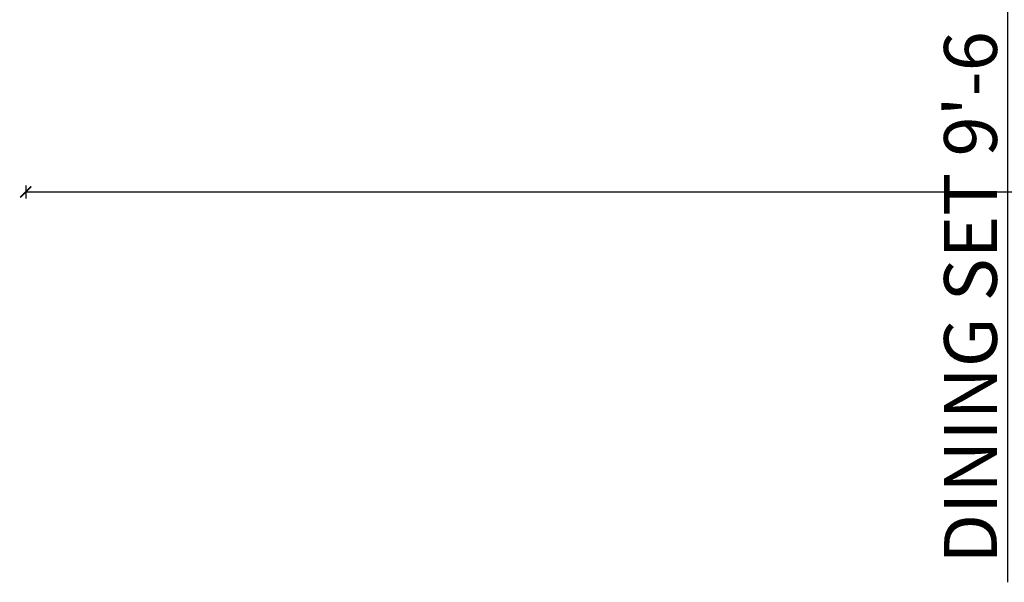
# Model space of a CAD drawing. Units: inches. Extents: x 375 to 1122, y 27 to 1069.
# Tile 1 of 155: x 443 to 667, y 27 to 155. Entities that reach past the tile are written whole.
import ezdxf

# ---------------------------------------------------------------- set-up
doc = ezdxf.new("R2010")
doc.units = ezdxf.units.IN
doc.layers.add('A-ANNO-DIMS', color=2, linetype='Continuous', lineweight=18)
doc.styles.get("Standard").update_dxf_attribs({"font": 'arial.ttf'})
doc.dimstyles.new('ISO-25', dxfattribs={"dimtxt": 12, "dimasz": 2.5, "dimexe": 1.5, "dimexo": 1.5, "dimtad": 1, "dimdec": 1, "dimlunit": 3, "dimtxsty": 'Standard', "dimblk": 'ARCHTICK', "dimcen": 2.5, "dimadec": 0, "dimazin": 0, "dimtfac": 1, "dimtdec": 1, "dimtmove": 0, "dimatfit": 3, "dimfxl": 1.5, "dimfxlon": 1, "dimarcsym": 0})

# ---------------------------------------------------------------- blocks, each defined once
blk = doc.blocks.new('_ArchTick')
at = {"color": 0, "linetype": 'ByBlock', "const_width": 0.15}
blk.add_lwpolyline([(-0.5, -0.5), (0.5, 0.5)], dxfattribs=at)
blk = doc.blocks.new('*D59')
at = {"layer": 'A-ANNO-DIMS', "color": 0, "lineweight": -2, "transparency": 16777216}
for p, q in [((668.72, 346.85), (665.72, 346.85)), ((667.22, 346.85), (667.22, 232.35)), ((668.72, 232.35), (665.72, 232.35)), ((667.22, 232.35), (667.22, 27.5))]:
    blk.add_line(p, q, dxfattribs=at)
at = {"layer": 'Defpoints', "color": 0, "transparency": 16777216}
for p in [(684.39, 346.85), (667.22, 232.35), (684.39, 232.35)]:
    blk.add_point(p, dxfattribs=at)
at = {"layer": 'A-ANNO-DIMS', "color": 0, "lineweight": -2, "transparency": 16777216, "xscale": 2.5, "yscale": 2.5, "zscale": 2.5}
for p, rotation in [((667.22, 346.85), 90), ((667.22, 232.35), 270)]:
    blk.add_blockref('_ArchTick', p, dxfattribs=dict(at, rotation=rotation))
at = {"layer": 'A-ANNO-DIMS', "color": 0, "transparency": 16777216, "insert": (660.39, 128.67), "char_height": 12, "attachment_point": 5, "rotation": 90}
blk.add_mtext('DINING SET 9\'-6 1/2" TYP.', dxfattribs=at)
blk = doc.blocks.new('*D81')
at = {"layer": 'A-ANNO-DIMS', "color": 0, "lineweight": -2, "transparency": 16777216}
for p, q in [((444.51, 117.53), (444.51, 114.53)), ((989.01, 117.53), (989.01, 114.53)), ((444.51, 116.03), (989.01, 116.03))]:
    blk.add_line(p, q, dxfattribs=at)
at = {"layer": 'Defpoints', "color": 0, "transparency": 16777216}
for p in [(444.51, 187.53), (989.01, 187.53), (989.01, 116.03)]:
    blk.add_point(p, dxfattribs=at)
at = {"layer": 'A-ANNO-DIMS', "color": 0, "lineweight": -2, "transparency": 16777216, "xscale": 2.5, "yscale": 2.5, "zscale": 2.5, "rotation": 180}
blk.add_blockref('_ArchTick', (444.51, 116.03), dxfattribs=at)
at = {"layer": 'A-ANNO-DIMS', "color": 0, "lineweight": -2, "transparency": 16777216, "xscale": 2.5, "yscale": 2.5, "zscale": 2.5}
blk.add_blockref('_ArchTick', (989.01, 116.03), dxfattribs=at)
at = {"layer": 'A-ANNO-DIMS', "color": 0, "transparency": 16777216, "insert": (716.76, 122.86), "char_height": 12, "attachment_point": 5}
blk.add_mtext('45\'-4 1/2"', dxfattribs=at)

msp = doc.modelspace()

# ---------------------------------------------------------------- dimensions: what is measured, and where the dimension line sits
at = {"layer": 'A-ANNO-DIMS'}
dim = msp.add_linear_dim(base=(667.22, 232.35), p1=(684.39, 346.85), p2=(684.39, 232.35), angle=270, text='DINING SET <> TYP.', dimstyle='ISO-25', override={"dimdec": 1, "dimlfac": 1, "dimrnd": 0, "dimzin": 1, "dimdsep": 46, "dimlunit": 4, "dimfrac": 2}, dxfattribs=at)
dim.commit()
dim.dimension.update_dxf_attribs({"geometry": '*D59', "text_midpoint": (660.39, 128.67)})
dim = msp.add_linear_dim(base=(989.01, 116.03), p1=(444.51, 187.53), p2=(989.01, 187.53), dimstyle='ISO-25', override={"dimdec": 1, "dimlfac": 1, "dimrnd": 0, "dimzin": 1, "dimdsep": 46, "dimlunit": 4, "dimfrac": 2}, dxfattribs=at)
dim.commit()
dim.dimension.update_dxf_attribs({"geometry": '*D81', "text_midpoint": (716.76, 122.86)})

doc.saveas('drawing.dxf')
